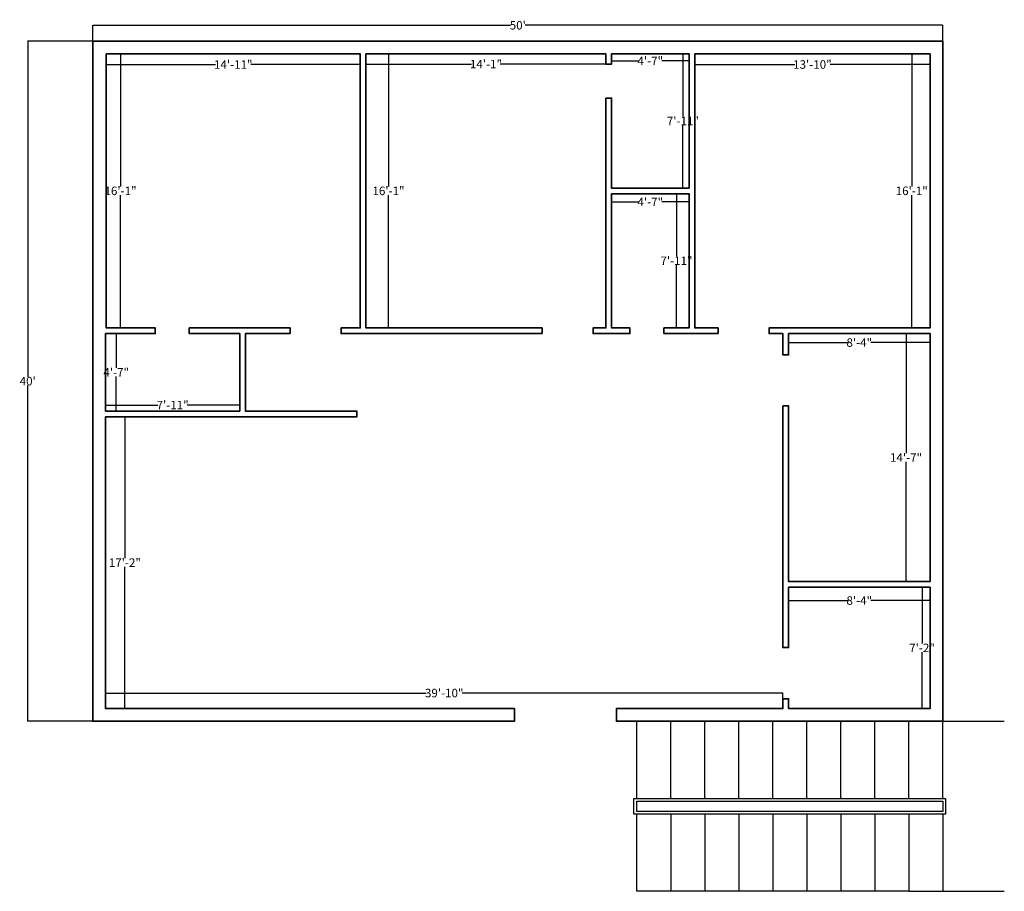
# Model space of a CAD drawing. Units: feet. Extents: x 3511 to 6270, y 2172 to 4127.
# Tile 4 of 4: x 5172 to 5867, y 3449 to 4064. Entities that reach past the tile are written whole.
import ezdxf

# ---------------------------------------------------------------- set-up
doc = ezdxf.new("R2010")
doc.units = ezdxf.units.FT
for name, color, linetype, lineweight in [('A-ANNO-DIMS', 2, 'Continuous', 18), ('A-FLOR-STRS', 4, 'Continuous', 25), ('A-WALL', 7, 'Continuous', 35)]:
    doc.layers.add(name, color=color, linetype=linetype, lineweight=lineweight)
doc.styles.get("Standard").update_dxf_attribs({"font": 'arial.ttf'})
doc.dimstyles.get("Standard").update_dxf_attribs({"dimtxt": 6, "dimasz": 0.18, "dimexe": 0.18, "dimexo": 0.0625, "dimgap": 0.09, "dimtad": 0, "dimtih": 1, "dimtoh": 1, "dimdec": 0, "dimzin": 0, "dimdsep": 46, "dimlunit": 3, "dimtxsty": 'Standard', "dimcen": 0.09, "dimadec": 0, "dimazin": 0, "dimtfac": 1, "dimtdec": 0, "dimtofl": 0, "dimtmove": 0, "dimatfit": 3, "dimfxl": 1, "dimtolj": 1, "dimtzin": 0, "dimarcsym": 0})

# ---------------------------------------------------------------- blocks, each defined once
blk = doc.blocks.new('*D52')
at = {"layer": 'A-ANNO-DIMS', "color": 0, "lineweight": -2, "transparency": 16777216}
for p, q in [((5232.7, 4039.51), (5232.7, 4031.86)), ((5412.04, 4039.51), (5412.04, 4031.86)), ((5232.88, 4032.04), (5309.93, 4032.04)), ((5411.86, 4032.04), (5334.82, 4032.04))]:
    blk.add_line(p, q, dxfattribs=at)
at = {"layer": 'A-ANNO-DIMS', "color": 0, "transparency": 16777216}
for points in [[(5232.88, 4032.07), (5232.88, 4032.01), (5232.7, 4032.04)], [(5411.86, 4032.07), (5411.86, 4032.01), (5412.04, 4032.04)]]:
    blk.add_solid(points, dxfattribs=at)
at = {"layer": 'Defpoints', "color": 0, "transparency": 16777216}
for p in [(5232.7, 4039.58), (5412.04, 4039.58), (5412.04, 4032.04)]:
    blk.add_point(p, dxfattribs=at)
at = {"layer": 'A-ANNO-DIMS', "color": 0, "transparency": 16777216, "insert": (5322.37, 4032.04), "char_height": 6, "attachment_point": 5}
blk.add_mtext('\\A1;14\'-11"', dxfattribs=at)
blk = doc.blocks.new('*D43')
at = {"layer": 'A-ANNO-DIMS', "color": 0, "lineweight": -2, "transparency": 16777216}
for p, q in [((5232.76, 4039.58), (5242.98, 4039.58)), ((5242.8, 4039.4), (5242.8, 3946.05)), ((5242.8, 3846.39), (5242.8, 3939.74)), ((5232.76, 3846.21), (5242.98, 3846.21))]:
    blk.add_line(p, q, dxfattribs=at)
at = {"layer": 'A-ANNO-DIMS', "color": 0, "transparency": 16777216}
for points in [[(5242.77, 4039.4), (5242.83, 4039.4), (5242.8, 4039.58)], [(5242.77, 3846.39), (5242.83, 3846.39), (5242.8, 3846.21)]]:
    blk.add_solid(points, dxfattribs=at)
at = {"layer": 'Defpoints', "color": 0, "transparency": 16777216}
for p in [(5232.7, 4039.58), (5232.7, 3846.21), (5242.8, 3846.21)]:
    blk.add_point(p, dxfattribs=at)
at = {"layer": 'A-ANNO-DIMS', "color": 0, "transparency": 16777216, "insert": (5242.8, 3942.89), "char_height": 6, "attachment_point": 5}
blk.add_mtext('\\A1;16\'-1"', dxfattribs=at)
blk = doc.blocks.new('*D44')
at = {"layer": 'A-ANNO-DIMS', "color": 0, "lineweight": -2, "transparency": 16777216}
for p, q in [((5416.04, 4039.51), (5416.04, 4032.14)), ((5585.38, 4039.51), (5585.38, 4032.14)), ((5416.22, 4032.32), (5490.6, 4032.32)), ((5585.2, 4032.32), (5510.82, 4032.32))]:
    blk.add_line(p, q, dxfattribs=at)
at = {"layer": 'A-ANNO-DIMS', "color": 0, "transparency": 16777216}
for points in [[(5416.22, 4032.35), (5416.22, 4032.29), (5416.04, 4032.32)], [(5585.2, 4032.35), (5585.2, 4032.29), (5585.38, 4032.32)]]:
    blk.add_solid(points, dxfattribs=at)
at = {"layer": 'Defpoints', "color": 0, "transparency": 16777216}
for p in [(5416.04, 4039.58), (5585.38, 4039.58), (5585.38, 4032.32)]:
    blk.add_point(p, dxfattribs=at)
at = {"layer": 'A-ANNO-DIMS', "color": 0, "transparency": 16777216, "insert": (5500.71, 4032.32), "char_height": 6, "attachment_point": 5}
blk.add_mtext('\\A1;14\'-1"', dxfattribs=at)
blk = doc.blocks.new('*D45')
at = {"layer": 'A-ANNO-DIMS', "color": 0, "lineweight": -2, "transparency": 16777216}
for p, q in [((5416.11, 4039.58), (5432.14, 4039.58)), ((5431.96, 4039.4), (5431.96, 3946.05)), ((5431.96, 3846.39), (5431.96, 3939.74)), ((5416.11, 3846.21), (5432.14, 3846.21))]:
    blk.add_line(p, q, dxfattribs=at)
at = {"layer": 'A-ANNO-DIMS', "color": 0, "transparency": 16777216}
for points in [[(5431.93, 4039.4), (5431.99, 4039.4), (5431.96, 4039.58)], [(5431.93, 3846.39), (5431.99, 3846.39), (5431.96, 3846.21)]]:
    blk.add_solid(points, dxfattribs=at)
at = {"layer": 'Defpoints', "color": 0, "transparency": 16777216}
for p in [(5416.04, 4039.58), (5416.04, 3846.21), (5431.96, 3846.21)]:
    blk.add_point(p, dxfattribs=at)
at = {"layer": 'A-ANNO-DIMS', "color": 0, "transparency": 16777216, "insert": (5431.96, 3942.89), "char_height": 6, "attachment_point": 5}
blk.add_mtext('\\A1;16\'-1"', dxfattribs=at)
blk = doc.blocks.new('*D46')
at = {"layer": 'A-ANNO-DIMS', "color": 0, "lineweight": -2, "transparency": 16777216}
for p, q in [((5589.38, 4039.51), (5589.38, 4034.45)), ((5644.08, 4039.51), (5644.08, 4034.45)), ((5589.56, 4034.63), (5608.54, 4034.63)), ((5643.9, 4034.63), (5624.91, 4034.63))]:
    blk.add_line(p, q, dxfattribs=at)
at = {"layer": 'A-ANNO-DIMS', "color": 0, "transparency": 16777216}
for points in [[(5589.56, 4034.66), (5589.56, 4034.6), (5589.38, 4034.63)], [(5643.9, 4034.66), (5643.9, 4034.6), (5644.08, 4034.63)]]:
    blk.add_solid(points, dxfattribs=at)
at = {"layer": 'Defpoints', "color": 0, "transparency": 16777216}
for p in [(5589.38, 4039.58), (5644.08, 4039.58), (5644.08, 4034.63)]:
    blk.add_point(p, dxfattribs=at)
at = {"layer": 'A-ANNO-DIMS', "color": 0, "transparency": 16777216, "insert": (5616.73, 4034.63), "char_height": 6, "attachment_point": 5}
blk.add_mtext('\\A1;4\'-7"', dxfattribs=at)
blk = doc.blocks.new('*D47')
at = {"layer": 'A-ANNO-DIMS', "color": 0, "lineweight": -2, "transparency": 16777216}
for p, q in [((5644.02, 4039.58), (5639.56, 4039.58)), ((5639.74, 4039.4), (5639.74, 3995.34)), ((5639.74, 3945.07), (5639.74, 3989.13)), ((5644.02, 3944.89), (5639.56, 3944.89))]:
    blk.add_line(p, q, dxfattribs=at)
at = {"layer": 'A-ANNO-DIMS', "color": 0, "transparency": 16777216}
for points in [[(5639.71, 4039.4), (5639.77, 4039.4), (5639.74, 4039.58)], [(5639.71, 3945.07), (5639.77, 3945.07), (5639.74, 3944.89)]]:
    blk.add_solid(points, dxfattribs=at)
at = {"layer": 'Defpoints', "color": 0, "transparency": 16777216}
for p in [(5644.08, 4039.58), (5639.74, 3944.89), (5644.08, 3944.89)]:
    blk.add_point(p, dxfattribs=at)
at = {"layer": 'A-ANNO-DIMS', "color": 0, "transparency": 16777216, "insert": (5639.74, 3992.23), "char_height": 6, "attachment_point": 5}
blk.add_mtext('\\A1;7\'-11"', dxfattribs=at)
blk = doc.blocks.new('*D48')
at = {"layer": 'A-ANNO-DIMS', "color": 0, "lineweight": -2, "transparency": 16777216}
for p, q in [((5648.08, 4039.51), (5648.08, 4031.89)), ((5814.21, 4039.51), (5814.21, 4031.89)), ((5648.26, 4032.07), (5718.7, 4032.07)), ((5814.03, 4032.07), (5743.59, 4032.07))]:
    blk.add_line(p, q, dxfattribs=at)
at = {"layer": 'A-ANNO-DIMS', "color": 0, "transparency": 16777216}
for points in [[(5648.26, 4032.1), (5648.26, 4032.04), (5648.08, 4032.07)], [(5814.03, 4032.1), (5814.03, 4032.04), (5814.21, 4032.07)]]:
    blk.add_solid(points, dxfattribs=at)
at = {"layer": 'Defpoints', "color": 0, "transparency": 16777216}
for p in [(5648.08, 4039.58), (5814.21, 4039.58), (5814.21, 4032.07)]:
    blk.add_point(p, dxfattribs=at)
at = {"layer": 'A-ANNO-DIMS', "color": 0, "transparency": 16777216, "insert": (5731.15, 4032.07), "char_height": 6, "attachment_point": 5}
blk.add_mtext('\\A1;13\'-10"', dxfattribs=at)
blk = doc.blocks.new('*D49')
at = {"layer": 'A-ANNO-DIMS', "color": 0, "lineweight": -2, "transparency": 16777216}
for p, q in [((5814.15, 4039.58), (5801.1, 4039.58)), ((5801.28, 4039.4), (5801.28, 3946.05)), ((5801.28, 3846.39), (5801.28, 3939.74)), ((5814.15, 3846.21), (5801.1, 3846.21))]:
    blk.add_line(p, q, dxfattribs=at)
at = {"layer": 'A-ANNO-DIMS', "color": 0, "transparency": 16777216}
for points in [[(5801.25, 4039.4), (5801.31, 4039.4), (5801.28, 4039.58)], [(5801.25, 3846.39), (5801.31, 3846.39), (5801.28, 3846.21)]]:
    blk.add_solid(points, dxfattribs=at)
at = {"layer": 'Defpoints', "color": 0, "transparency": 16777216}
for p in [(5814.21, 4039.58), (5801.28, 3846.21), (5814.21, 3846.21)]:
    blk.add_point(p, dxfattribs=at)
at = {"layer": 'A-ANNO-DIMS', "color": 0, "transparency": 16777216, "insert": (5801.28, 3942.89), "char_height": 6, "attachment_point": 5}
blk.add_mtext('\\A1;16\'-1"', dxfattribs=at)
blk = doc.blocks.new('*D50')
at = {"layer": 'A-ANNO-DIMS', "color": 0, "lineweight": -2, "transparency": 16777216}
for p, q in [((5644.02, 3940.89), (5635.02, 3940.89)), ((5635.2, 3940.71), (5635.2, 3896.65)), ((5635.2, 3846.39), (5635.2, 3890.45)), ((5644.02, 3846.21), (5635.02, 3846.21))]:
    blk.add_line(p, q, dxfattribs=at)
at = {"layer": 'A-ANNO-DIMS', "color": 0, "transparency": 16777216}
for points in [[(5635.17, 3940.71), (5635.23, 3940.71), (5635.2, 3940.89)], [(5635.17, 3846.39), (5635.23, 3846.39), (5635.2, 3846.21)]]:
    blk.add_solid(points, dxfattribs=at)
at = {"layer": 'Defpoints', "color": 0, "transparency": 16777216}
for p in [(5644.08, 3940.89), (5635.2, 3846.21), (5644.08, 3846.21)]:
    blk.add_point(p, dxfattribs=at)
at = {"layer": 'A-ANNO-DIMS', "color": 0, "transparency": 16777216, "insert": (5635.2, 3893.55), "char_height": 6, "attachment_point": 5}
blk.add_mtext('\\A1;7\'-11"', dxfattribs=at)
blk = doc.blocks.new('*D51')
at = {"layer": 'A-ANNO-DIMS', "color": 0, "lineweight": -2, "transparency": 16777216}
for p, q in [((5589.38, 3940.83), (5589.38, 3934.92)), ((5644.08, 3940.83), (5644.08, 3934.92)), ((5589.56, 3935.1), (5608.54, 3935.1)), ((5643.9, 3935.1), (5624.91, 3935.1))]:
    blk.add_line(p, q, dxfattribs=at)
at = {"layer": 'A-ANNO-DIMS', "color": 0, "transparency": 16777216}
for points in [[(5589.56, 3935.13), (5589.56, 3935.07), (5589.38, 3935.1)], [(5643.9, 3935.13), (5643.9, 3935.07), (5644.08, 3935.1)]]:
    blk.add_solid(points, dxfattribs=at)
at = {"layer": 'Defpoints', "color": 0, "transparency": 16777216}
for p in [(5589.38, 3940.89), (5644.08, 3940.89), (5644.08, 3935.1)]:
    blk.add_point(p, dxfattribs=at)
at = {"layer": 'A-ANNO-DIMS', "color": 0, "transparency": 16777216, "insert": (5616.73, 3935.1), "char_height": 6, "attachment_point": 5}
blk.add_mtext('\\A1;4\'-7"', dxfattribs=at)
blk = doc.blocks.new('*D53')
at = {"layer": 'A-ANNO-DIMS', "color": 0, "lineweight": -2, "transparency": 16777216}
for p, q in [((5232.21, 3787.57), (5232.21, 3791.87)), ((5232.39, 3791.69), (5269.18, 3791.69)), ((5326.72, 3791.69), (5289.93, 3791.69)), ((5326.9, 3787.57), (5326.9, 3791.87))]:
    blk.add_line(p, q, dxfattribs=at)
at = {"layer": 'A-ANNO-DIMS', "color": 0, "transparency": 16777216}
for points in [[(5232.39, 3791.72), (5232.39, 3791.66), (5232.21, 3791.69)], [(5326.72, 3791.72), (5326.72, 3791.66), (5326.9, 3791.69)]]:
    blk.add_solid(points, dxfattribs=at)
at = {"layer": 'Defpoints', "color": 0, "transparency": 16777216}
for p in [(5326.9, 3791.69), (5232.21, 3787.5), (5326.9, 3787.5)]:
    blk.add_point(p, dxfattribs=at)
at = {"layer": 'A-ANNO-DIMS', "color": 0, "transparency": 16777216, "insert": (5279.56, 3791.69), "char_height": 6, "attachment_point": 5}
blk.add_mtext('\\A1;7\'-11"', dxfattribs=at)
blk = doc.blocks.new('*D54')
at = {"layer": 'A-ANNO-DIMS', "color": 0, "lineweight": -2, "transparency": 16777216}
for p, q in [((5232.28, 3842.21), (5239.91, 3842.21)), ((5239.73, 3842.03), (5239.73, 3817.95)), ((5239.73, 3787.68), (5239.73, 3811.77)), ((5232.28, 3787.5), (5239.91, 3787.5))]:
    blk.add_line(p, q, dxfattribs=at)
at = {"layer": 'A-ANNO-DIMS', "color": 0, "transparency": 16777216}
for points in [[(5239.7, 3842.03), (5239.76, 3842.03), (5239.73, 3842.21)], [(5239.7, 3787.68), (5239.76, 3787.68), (5239.73, 3787.5)]]:
    blk.add_solid(points, dxfattribs=at)
at = {"layer": 'Defpoints', "color": 0, "transparency": 16777216}
for p in [(5232.21, 3842.21), (5239.73, 3842.21), (5232.21, 3787.5)]:
    blk.add_point(p, dxfattribs=at)
at = {"layer": 'A-ANNO-DIMS', "color": 0, "transparency": 16777216, "insert": (5239.73, 3814.86), "char_height": 6, "attachment_point": 5}
blk.add_mtext('\\A1;4\'-7"', dxfattribs=at)
blk = doc.blocks.new('*D55')
at = {"layer": 'A-ANNO-DIMS', "color": 0, "lineweight": -2, "transparency": 16777216}
for p, q in [((5232.21, 3577.64), (5232.21, 3588.67)), ((5232.39, 3588.49), (5458.53, 3588.49)), ((5710.12, 3588.49), (5483.98, 3588.49)), ((5710.3, 3577.64), (5710.3, 3588.67))]:
    blk.add_line(p, q, dxfattribs=at)
at = {"layer": 'A-ANNO-DIMS', "color": 0, "transparency": 16777216}
for points in [[(5232.39, 3588.52), (5232.39, 3588.46), (5232.21, 3588.49)], [(5710.12, 3588.52), (5710.12, 3588.46), (5710.3, 3588.49)]]:
    blk.add_solid(points, dxfattribs=at)
at = {"layer": 'Defpoints', "color": 0, "transparency": 16777216}
for p in [(5710.3, 3588.49), (5232.21, 3577.58), (5710.3, 3577.58)]:
    blk.add_point(p, dxfattribs=at)
at = {"layer": 'A-ANNO-DIMS', "color": 0, "transparency": 16777216, "insert": (5471.26, 3588.49), "char_height": 6, "attachment_point": 5}
blk.add_mtext('\\A1;39\'-10"', dxfattribs=at)
blk = doc.blocks.new('*D56')
at = {"layer": 'A-ANNO-DIMS', "color": 0, "lineweight": -2, "transparency": 16777216}
for p, q in [((5232.28, 3783.5), (5246.03, 3783.5)), ((5245.85, 3783.32), (5245.85, 3683.64)), ((5245.85, 3577.76), (5245.85, 3677.44)), ((5232.28, 3577.58), (5246.03, 3577.58))]:
    blk.add_line(p, q, dxfattribs=at)
at = {"layer": 'A-ANNO-DIMS', "color": 0, "transparency": 16777216}
for points in [[(5245.82, 3783.32), (5245.88, 3783.32), (5245.85, 3783.5)], [(5245.82, 3577.76), (5245.88, 3577.76), (5245.85, 3577.58)]]:
    blk.add_solid(points, dxfattribs=at)
at = {"layer": 'Defpoints', "color": 0, "transparency": 16777216}
for p in [(5232.21, 3783.5), (5232.21, 3577.58), (5245.85, 3577.58)]:
    blk.add_point(p, dxfattribs=at)
at = {"layer": 'A-ANNO-DIMS', "color": 0, "transparency": 16777216, "insert": (5245.85, 3680.54), "char_height": 6, "attachment_point": 5}
blk.add_mtext('\\A1;17\'-2"', dxfattribs=at)
blk = doc.blocks.new('*D57')
at = {"layer": 'A-ANNO-DIMS', "color": 0, "lineweight": -2, "transparency": 16777216}
for p, q in [((5814.15, 3842.21), (5797.07, 3842.21)), ((5797.25, 3842.03), (5797.25, 3757.78)), ((5797.25, 3667.33), (5797.25, 3751.57)), ((5814.15, 3667.15), (5797.07, 3667.15))]:
    blk.add_line(p, q, dxfattribs=at)
at = {"layer": 'A-ANNO-DIMS', "color": 0, "transparency": 16777216}
for points in [[(5797.22, 3842.03), (5797.28, 3842.03), (5797.25, 3842.21)], [(5797.22, 3667.33), (5797.28, 3667.33), (5797.25, 3667.15)]]:
    blk.add_solid(points, dxfattribs=at)
at = {"layer": 'Defpoints', "color": 0, "transparency": 16777216}
for p in [(5814.21, 3842.21), (5797.25, 3667.15), (5814.21, 3667.15)]:
    blk.add_point(p, dxfattribs=at)
at = {"layer": 'A-ANNO-DIMS', "color": 0, "transparency": 16777216, "insert": (5797.25, 3754.68), "char_height": 6, "attachment_point": 5}
blk.add_mtext('\\A1;14\'-7"', dxfattribs=at)
blk = doc.blocks.new('*D58')
at = {"layer": 'A-ANNO-DIMS', "color": 0, "lineweight": -2, "transparency": 16777216}
for p, q in [((5714.3, 3842.15), (5714.3, 3835.65)), ((5814.21, 3842.15), (5814.21, 3835.65)), ((5714.48, 3835.83), (5756.19, 3835.83)), ((5814.03, 3835.83), (5772.33, 3835.83))]:
    blk.add_line(p, q, dxfattribs=at)
at = {"layer": 'A-ANNO-DIMS', "color": 0, "transparency": 16777216}
for points in [[(5714.48, 3835.86), (5714.48, 3835.8), (5714.3, 3835.83)], [(5814.03, 3835.86), (5814.03, 3835.8), (5814.21, 3835.83)]]:
    blk.add_solid(points, dxfattribs=at)
at = {"layer": 'Defpoints', "color": 0, "transparency": 16777216}
for p in [(5714.3, 3842.21), (5814.21, 3842.21), (5714.3, 3835.83)]:
    blk.add_point(p, dxfattribs=at)
at = {"layer": 'A-ANNO-DIMS', "color": 0, "transparency": 16777216, "insert": (5764.26, 3835.83), "char_height": 6, "attachment_point": 5}
blk.add_mtext('\\A1;8\'-4"', dxfattribs=at)
blk = doc.blocks.new('*D59')
at = {"layer": 'A-ANNO-DIMS', "color": 0, "lineweight": -2, "transparency": 16777216}
for p, q in [((5814.15, 3663.15), (5808.38, 3663.15)), ((5808.56, 3662.97), (5808.56, 3623.46)), ((5808.56, 3577.76), (5808.56, 3617.26)), ((5814.15, 3577.58), (5808.38, 3577.58))]:
    blk.add_line(p, q, dxfattribs=at)
at = {"layer": 'A-ANNO-DIMS', "color": 0, "transparency": 16777216}
for points in [[(5808.53, 3662.97), (5808.59, 3662.97), (5808.56, 3663.15)], [(5808.53, 3577.76), (5808.59, 3577.76), (5808.56, 3577.58)]]:
    blk.add_solid(points, dxfattribs=at)
at = {"layer": 'Defpoints', "color": 0, "transparency": 16777216}
for p in [(5814.21, 3663.15), (5808.56, 3577.58), (5814.21, 3577.58)]:
    blk.add_point(p, dxfattribs=at)
at = {"layer": 'A-ANNO-DIMS', "color": 0, "transparency": 16777216, "insert": (5808.56, 3620.36), "char_height": 6, "attachment_point": 5}
blk.add_mtext('\\A1;7\'-2"', dxfattribs=at)
blk = doc.blocks.new('*D60')
at = {"layer": 'A-ANNO-DIMS', "color": 0, "lineweight": -2, "transparency": 16777216}
for p, q in [((5714.3, 3663.08), (5714.3, 3653.6)), ((5814.21, 3663.08), (5814.21, 3653.6)), ((5714.48, 3653.78), (5756.19, 3653.78)), ((5814.03, 3653.78), (5772.33, 3653.78))]:
    blk.add_line(p, q, dxfattribs=at)
at = {"layer": 'A-ANNO-DIMS', "color": 0, "transparency": 16777216}
for points in [[(5714.48, 3653.81), (5714.48, 3653.75), (5714.3, 3653.78)], [(5814.03, 3653.81), (5814.03, 3653.75), (5814.21, 3653.78)]]:
    blk.add_solid(points, dxfattribs=at)
at = {"layer": 'Defpoints', "color": 0, "transparency": 16777216}
for p in [(5714.3, 3663.15), (5814.21, 3663.15), (5714.3, 3653.78)]:
    blk.add_point(p, dxfattribs=at)
at = {"layer": 'A-ANNO-DIMS', "color": 0, "transparency": 16777216, "insert": (5764.26, 3653.78), "char_height": 6, "attachment_point": 5}
blk.add_mtext('\\A1;8\'-4"', dxfattribs=at)
blk = doc.blocks.new('*D61')
at = {"layer": 'A-ANNO-DIMS', "color": 0, "lineweight": -2, "transparency": 16777216}
for p, q in [((5223.15, 4048.58), (5177.1, 4048.58)), ((5177.28, 4048.4), (5177.28, 3811.73)), ((5177.28, 3568.76), (5177.28, 3805.42)), ((5223.15, 3568.58), (5177.1, 3568.58))]:
    blk.add_line(p, q, dxfattribs=at)
at = {"layer": 'A-ANNO-DIMS', "color": 0, "transparency": 16777216}
for points in [[(5177.25, 4048.4), (5177.31, 4048.4), (5177.28, 4048.58)], [(5177.25, 3568.76), (5177.31, 3568.76), (5177.28, 3568.58)]]:
    blk.add_solid(points, dxfattribs=at)
at = {"layer": 'Defpoints', "color": 0, "transparency": 16777216}
for p in [(5223.21, 4048.58), (5177.28, 3568.58), (5223.21, 3568.58)]:
    blk.add_point(p, dxfattribs=at)
at = {"layer": 'A-ANNO-DIMS', "color": 0, "transparency": 16777216, "insert": (5177.28, 3808.58), "char_height": 6, "attachment_point": 5}
blk.add_mtext("\\A1;40'", dxfattribs=at)
blk = doc.blocks.new('*D62')
at = {"layer": 'A-ANNO-DIMS', "color": 0, "lineweight": -2, "transparency": 16777216}
for p, q in [((5223.21, 4048.64), (5223.21, 4059.92)), ((5223.39, 4059.74), (5518.03, 4059.74)), ((5823.03, 4059.74), (5528.4, 4059.74)), ((5823.21, 4048.64), (5823.21, 4059.92))]:
    blk.add_line(p, q, dxfattribs=at)
at = {"layer": 'A-ANNO-DIMS', "color": 0, "transparency": 16777216}
for points in [[(5223.39, 4059.77), (5223.39, 4059.71), (5223.21, 4059.74)], [(5823.03, 4059.77), (5823.03, 4059.71), (5823.21, 4059.74)]]:
    blk.add_solid(points, dxfattribs=at)
at = {"layer": 'Defpoints', "color": 0, "transparency": 16777216}
for p in [(5823.21, 4059.74), (5223.21, 4048.58), (5823.21, 4048.58)]:
    blk.add_point(p, dxfattribs=at)
at = {"layer": 'A-ANNO-DIMS', "color": 0, "transparency": 16777216, "insert": (5523.21, 4059.74), "char_height": 6, "attachment_point": 5}
blk.add_mtext("\\A1;50'", dxfattribs=at)
blk = doc.blocks.new('STAIR')
for p, q in [((2, 65.57), (2, 120)), ((26, 65.57), (26, 120)), ((50, 65.57), (50, 120)), ((74, 65.57), (74, 120)), ((98, 65.57), (98, 120)), ((122, 65.57), (122, 120)), ((146, 65.57), (146, 120)), ((170, 65.57), (170, 120)), ((194, 65.57), (194, 120)), ((218, 54.42), (218, 0))]:
    blk.add_line(p, q)
for points in [[(218, 65.57), (218, 120), (261.4, 120)], [(26, 54.42), (26, 0), (14, 0), (2, 0), (2, 54.42)], [(50, 54.42), (50, 0), (38, 0), (26, 0)], [(74, 54.42), (74, 0), (62, 0), (50, 0)], [(98, 54.42), (98, 0), (86, 0), (74, 0)], [(122, 54.42), (122, 0), (110, 0), (98, 0)], [(146, 54.42), (146, 0), (134, 0), (122, 0)], [(170, 54.42), (170, 0), (158, 0), (146, 0)], [(194, 54.42), (194, 0), (182, 0), (170, 0)], [(194, 0), (206, 0), (218, 0), (261.4, 0)]]:
    blk.add_lwpolyline(points)
for points in [[(0, 65.57), (220, 65.57), (220, 54.42), (0, 54.42)], [(218, 56.42), (2, 56.42), (2, 63.57), (218, 63.57)]]:
    blk.add_lwpolyline(points, close=True)

msp = doc.modelspace()

# ---------------------------------------------------------------- linework, layer by layer
at = {"layer": 'A-WALL'}
msp.add_lwpolyline([(5714.3, 3663.15), (5714.3, 3620.52), (5710.3, 3620.52), (5710.3, 3791.14), (5714.3, 3791.14), (5714.3, 3667.15), (5814.21, 3667.15), (5814.21, 3842.21), (5714.3, 3842.21), (5714.3, 3827.14), (5710.3, 3827.14), (5710.3, 3842.21), (5700.62, 3842.21), (5700.62, 3846.21), (5814.21, 3846.21), (5814.21, 4039.58), (5648.08, 4039.58), (5648.08, 3846.21), (5664.62, 3846.21), (5664.62, 3842.21), (5626.31, 3842.21), (5626.31, 3846.21), (5644.08, 3846.21), (5644.08, 3940.89), (5589.38, 3940.89), (5589.38, 3846.21), (5602.31, 3846.21), (5602.31, 3842.21), (5576.38, 3842.21), (5576.38, 3846.21), (5585.38, 3846.21), (5585.38, 4008.32), (5589.38, 4008.32), (5589.38, 3944.89), (5644.08, 3944.89), (5644.08, 4039.58), (5589.38, 4039.58), (5589.38, 4032.32), (5585.38, 4032.32), (5585.38, 4039.58), (5416.04, 4039.58), (5416.04, 3846.21), (5540.38, 3846.21), (5540.38, 3842.21), (5398.48, 3842.21), (5398.48, 3846.21), (5412.04, 3846.21), (5412.04, 4039.58), (5232.7, 4039.58), (5232.7, 3846.21), (5267.23, 3846.21), (5267.23, 3842.21), (5232.21, 3842.21), (5232.21, 3787.5), (5232.21, 3787.5), (5326.9, 3787.5), (5326.9, 3842.21), (5291.23, 3842.21), (5291.23, 3846.21), (5362.48, 3846.21), (5362.48, 3842.21), (5330.9, 3842.21), (5330.9, 3787.51), (5409.65, 3787.51), (5409.65, 3783.5), (5232.21, 3783.5), (5232.21, 3577.58), (5520.86, 3577.58), (5520.86, 3568.58), (5223.21, 3568.58), (5223.21, 4048.58), (5823.21, 4048.58), (5823.21, 3568.58), (5592.86, 3568.58), (5592.86, 3577.58), (5710.3, 3577.58), (5710.3, 3584.52), (5714.3, 3584.52), (5714.3, 3577.58), (5814.21, 3577.58), (5814.21, 3663.15)], close=True, dxfattribs=at)
msp.add_lwpolyline([(5330.9, 3783.5), (5330.9, 3783.5)], dxfattribs=at)

# ---------------------------------------------------------------- block references
at = {"layer": 'A-FLOR-STRS'}
msp.add_blockref('STAIR', (5605.21, 3448.58), dxfattribs=at)

# ---------------------------------------------------------------- dimensions: what is measured, and where the dimension line sits
at = {"layer": 'A-ANNO-DIMS'}
for base, p1, p2, picture, middle in [((5823.21, 4059.74), (5223.21, 4048.58), (5823.21, 4048.58), '*D62', (5523.21, 4059.74)), ((5412.04, 4032.04), (5232.7, 4039.58), (5412.04, 4039.58), '*D52', (5322.37, 4032.04)), ((5585.38, 4032.32), (5416.04, 4039.58), (5585.38, 4039.58), '*D44', (5500.71, 4032.32)), ((5644.08, 4034.63), (5589.38, 4039.58), (5644.08, 4039.58), '*D46', (5616.73, 4034.63)), ((5814.21, 4032.07), (5648.08, 4039.58), (5814.21, 4039.58), '*D48', (5731.15, 4032.07)), ((5644.08, 3935.1), (5589.38, 3940.89), (5644.08, 3940.89), '*D51', (5616.73, 3935.1)), ((5714.3, 3835.83), (5814.21, 3842.21), (5714.3, 3842.21), '*D58', (5764.26, 3835.83)), ((5326.9, 3791.69), (5232.21, 3787.5), (5326.9, 3787.5), '*D53', (5279.56, 3791.69)), ((5714.3, 3653.78), (5814.21, 3663.15), (5714.3, 3663.15), '*D60', (5764.26, 3653.78)), ((5710.3, 3588.49), (5232.21, 3577.58), (5710.3, 3577.58), '*D55', (5471.26, 3588.49))]:
    dim = msp.add_linear_dim(base=base, p1=p1, p2=p2, dimstyle='Standard', override={"dimclrd": 0, "dimclre": 0, "dimclrt": 0}, dxfattribs=at)
    dim.commit()
    dim.dimension.update_dxf_attribs({"geometry": picture, "text_midpoint": middle})
for base, p1, p2, picture, middle in [((5177.28, 3568.58), (5223.21, 4048.58), (5223.21, 3568.58), '*D61', (5177.28, 3808.58)), ((5242.8, 3846.21), (5232.7, 4039.58), (5232.7, 3846.21), '*D43', (5242.8, 3942.89)), ((5431.96, 3846.21), (5416.04, 4039.58), (5416.04, 3846.21), '*D45', (5431.96, 3942.89)), ((5639.74, 3944.89), (5644.08, 4039.58), (5644.08, 3944.89), '*D47', (5639.74, 3992.23)), ((5801.28, 3846.21), (5814.21, 4039.58), (5814.21, 3846.21), '*D49', (5801.28, 3942.89)), ((5635.2, 3846.21), (5644.08, 3940.89), (5644.08, 3846.21), '*D50', (5635.2, 3893.55)), ((5239.73, 3842.21), (5232.21, 3787.5), (5232.21, 3842.21), '*D54', (5239.73, 3814.86)), ((5797.25, 3667.15), (5814.21, 3842.21), (5814.21, 3667.15), '*D57', (5797.25, 3754.68)), ((5245.85, 3577.58), (5232.21, 3783.5), (5232.21, 3577.58), '*D56', (5245.85, 3680.54)), ((5808.56, 3577.58), (5814.21, 3663.15), (5814.21, 3577.58), '*D59', (5808.56, 3620.36))]:
    dim = msp.add_linear_dim(base=base, p1=p1, p2=p2, angle=90, dimstyle='Standard', override={"dimclrd": 0, "dimclre": 0, "dimclrt": 0}, dxfattribs=at)
    dim.commit()
    dim.dimension.update_dxf_attribs({"geometry": picture, "text_midpoint": middle})

doc.saveas('drawing.dxf')
